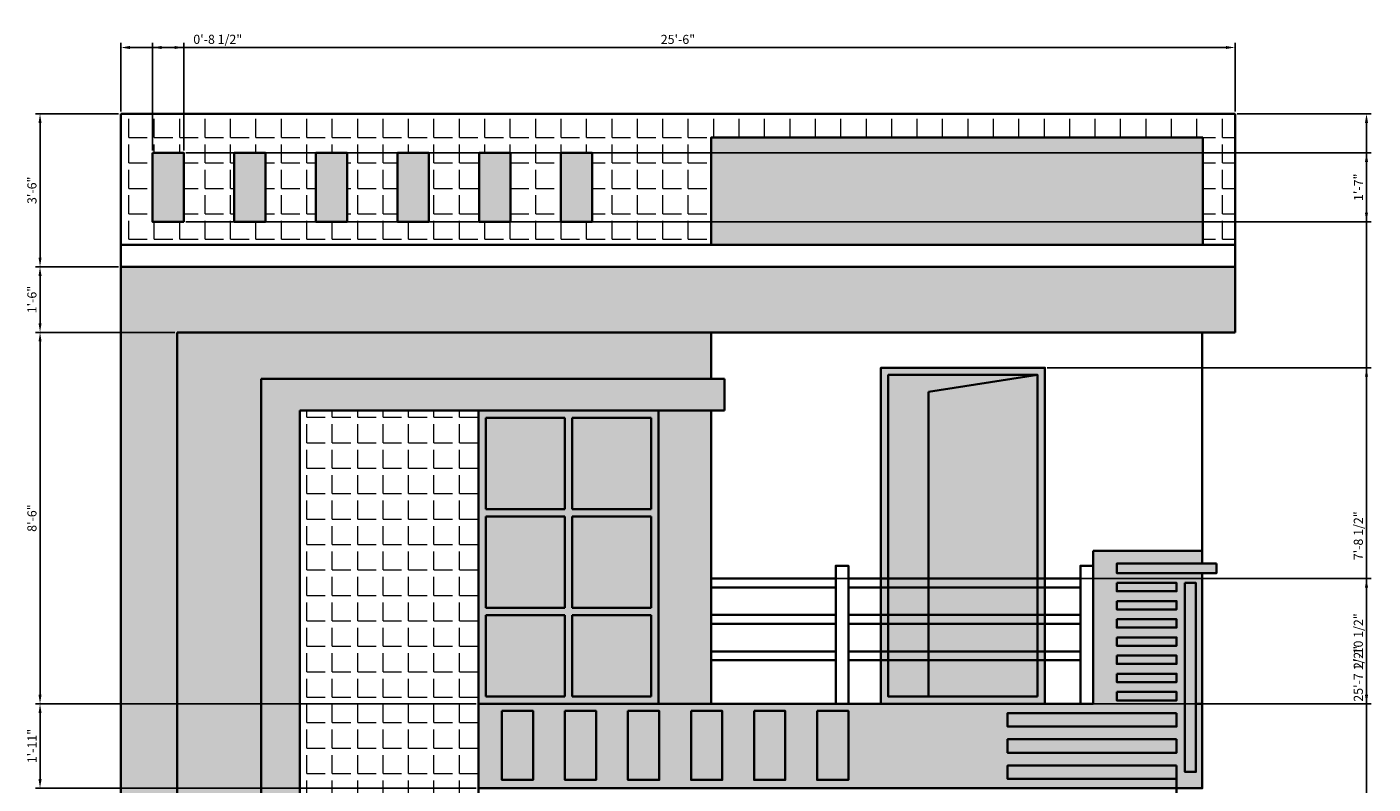
# Model space of a CAD drawing. Units: inches. Extents: x 2117 to 3047, y 1240 to 2266.
# Tile 3 of 4: x 2214 to 2584, y 2058 to 2266. Entities that reach past the tile are written whole.
import ezdxf

# ---------------------------------------------------------------- set-up
doc = ezdxf.new("R2010")
doc.units = ezdxf.units.IN
for name, color, linetype, lineweight in [('A-ANNO-DIMS', 2, 'Continuous', 18), ('A-ELEV', 7, 'Continuous', 35), ('A-ELEV-PATT', 8, 'Continuous', 13)]:
    doc.layers.add(name, color=color, linetype=linetype, lineweight=lineweight)
doc.styles.get("Standard").update_dxf_attribs({"font": 'arial.ttf'})
doc.dimstyles.new('ISO-25', dxfattribs={"dimtxt": 2.5, "dimasz": 2.5, "dimexe": 1.25, "dimexo": 0.625, "dimtad": 1, "dimdec": 1, "dimlunit": 3, "dimtxsty": 'Standard', "dimcen": 2.5, "dimadec": 0, "dimazin": 0, "dimtfac": 1, "dimtdec": 1, "dimtmove": 0, "dimatfit": 3, "dimfxl": 1, "dimarcsym": 0})
pattern_1 = [(0, (0, 0), (0, 6.985), [5.08, -1.905]), (90, (0, 0), (-6.985, 4e-16), [5.08, -1.905])]

# ---------------------------------------------------------------- blocks, each defined once
blk = doc.blocks.new('*D40')
at = {"layer": 'A-ANNO-DIMS', "color": 0, "lineweight": -2, "transparency": 16777216}
for p, q in [((2240.01, 2242.33), (2240.01, 2261.15)), ((2242.51, 2259.9), (2543.51, 2259.9)), ((2546.01, 2242.33), (2546.01, 2261.15))]:
    blk.add_line(p, q, dxfattribs=at)
at = {"layer": 'A-ANNO-DIMS', "color": 0, "transparency": 16777216}
for points in [[(2242.51, 2260.32), (2242.51, 2259.48), (2240.01, 2259.9)], [(2543.51, 2260.32), (2543.51, 2259.48), (2546.01, 2259.9)]]:
    blk.add_solid(points, dxfattribs=at)
at = {"layer": 'Defpoints', "color": 0, "transparency": 16777216}
for p in [(2546.01, 2259.9), (2240.01, 2241.7), (2546.01, 2241.7)]:
    blk.add_point(p, dxfattribs=at)
at = {"layer": 'A-ANNO-DIMS', "color": 0, "transparency": 16777216, "insert": (2393.01, 2261.8), "char_height": 2.5, "attachment_point": 5}
blk.add_mtext('25\'-6"', dxfattribs=at)
blk = doc.blocks.new('*D41')
at = {"layer": 'A-ANNO-DIMS', "color": 0, "lineweight": -2, "transparency": 16777216}
for p, q in [((2248.68, 2231.63), (2248.68, 2261.15)), ((2251.18, 2259.9), (2254.76, 2259.9)), ((2257.26, 2231.63), (2257.26, 2261.15)), ((2257.26, 2259.9), (2273.48, 2259.9))]:
    blk.add_line(p, q, dxfattribs=at)
at = {"layer": 'A-ANNO-DIMS', "color": 0, "transparency": 16777216}
for points in [[(2251.18, 2260.32), (2251.18, 2259.48), (2248.68, 2259.9)], [(2254.76, 2260.32), (2254.76, 2259.48), (2257.26, 2259.9)]]:
    blk.add_solid(points, dxfattribs=at)
at = {"layer": 'Defpoints', "color": 0, "transparency": 16777216}
for p in [(2257.26, 2259.9), (2248.68, 2231), (2257.26, 2231)]:
    blk.add_point(p, dxfattribs=at)
at = {"layer": 'A-ANNO-DIMS', "color": 0, "transparency": 16777216, "insert": (2266.62, 2261.82), "char_height": 2.5, "attachment_point": 5}
blk.add_mtext('0\'-8 1/2"', dxfattribs=at)
blk = doc.blocks.new('*D44')
at = {"layer": 'A-ANNO-DIMS', "color": 0, "lineweight": -2, "transparency": 16777216}
for p, q in [((2337.6, 2079.7), (2216.56, 2079.7)), ((2217.81, 2059.04), (2217.81, 2077.2)), ((2337.6, 2056.54), (2216.56, 2056.54))]:
    blk.add_line(p, q, dxfattribs=at)
at = {"layer": 'A-ANNO-DIMS', "color": 0, "transparency": 16777216}
for points in [[(2217.4, 2077.2), (2218.23, 2077.2), (2217.81, 2079.7)], [(2217.4, 2059.04), (2218.23, 2059.04), (2217.81, 2056.54)]]:
    blk.add_solid(points, dxfattribs=at)
at = {"layer": 'Defpoints', "color": 0, "transparency": 16777216}
for p in [(2217.81, 2079.7), (2338.23, 2079.7), (2338.23, 2056.54)]:
    blk.add_point(p, dxfattribs=at)
at = {"layer": 'A-ANNO-DIMS', "color": 0, "transparency": 16777216, "insert": (2215.93, 2068.12), "char_height": 2.5, "attachment_point": 5, "rotation": 90}
blk.add_mtext('1\'-11"', dxfattribs=at)
blk = doc.blocks.new('*D45')
at = {"layer": 'A-ANNO-DIMS', "color": 0, "lineweight": -2, "transparency": 16777216}
for p, q in [((2254.8, 2181.7), (2216.56, 2181.7)), ((2217.81, 2082.2), (2217.81, 2179.2)), ((2337.6, 2079.7), (2216.56, 2079.7))]:
    blk.add_line(p, q, dxfattribs=at)
at = {"layer": 'A-ANNO-DIMS', "color": 0, "transparency": 16777216}
for points in [[(2217.4, 2179.2), (2218.23, 2179.2), (2217.81, 2181.7)], [(2217.4, 2082.2), (2218.23, 2082.2), (2217.81, 2079.7)]]:
    blk.add_solid(points, dxfattribs=at)
at = {"layer": 'Defpoints', "color": 0, "transparency": 16777216}
for p in [(2217.81, 2181.7), (2255.43, 2181.7), (2338.23, 2079.7)]:
    blk.add_point(p, dxfattribs=at)
at = {"layer": 'A-ANNO-DIMS', "color": 0, "transparency": 16777216, "insert": (2215.91, 2130.7), "char_height": 2.5, "attachment_point": 5, "rotation": 90}
blk.add_mtext('8\'-6"', dxfattribs=at)
blk = doc.blocks.new('*D46')
at = {"layer": 'A-ANNO-DIMS', "color": 0, "lineweight": -2, "transparency": 16777216}
for p, q in [((2239.39, 2199.7), (2216.56, 2199.7)), ((2217.81, 2184.2), (2217.81, 2197.2)), ((2254.8, 2181.7), (2216.56, 2181.7))]:
    blk.add_line(p, q, dxfattribs=at)
at = {"layer": 'A-ANNO-DIMS', "color": 0, "transparency": 16777216}
for points in [[(2217.4, 2197.2), (2218.23, 2197.2), (2217.81, 2199.7)], [(2217.4, 2184.2), (2218.23, 2184.2), (2217.81, 2181.7)]]:
    blk.add_solid(points, dxfattribs=at)
at = {"layer": 'Defpoints', "color": 0, "transparency": 16777216}
for p in [(2217.81, 2199.7), (2240.01, 2199.7), (2255.43, 2181.7)]:
    blk.add_point(p, dxfattribs=at)
at = {"layer": 'A-ANNO-DIMS', "color": 0, "transparency": 16777216, "insert": (2215.91, 2190.7), "char_height": 2.5, "attachment_point": 5, "rotation": 90}
blk.add_mtext('1\'-6"', dxfattribs=at)
blk = doc.blocks.new('*D47')
at = {"layer": 'A-ANNO-DIMS', "color": 0, "lineweight": -2, "transparency": 16777216}
for p, q in [((2239.39, 2241.7), (2216.56, 2241.7)), ((2217.81, 2202.2), (2217.81, 2239.2)), ((2239.39, 2199.7), (2216.56, 2199.7))]:
    blk.add_line(p, q, dxfattribs=at)
at = {"layer": 'A-ANNO-DIMS', "color": 0, "transparency": 16777216}
for points in [[(2217.4, 2239.2), (2218.23, 2239.2), (2217.81, 2241.7)], [(2217.4, 2202.2), (2218.23, 2202.2), (2217.81, 2199.7)]]:
    blk.add_solid(points, dxfattribs=at)
at = {"layer": 'Defpoints', "color": 0, "transparency": 16777216}
for p in [(2217.81, 2241.7), (2240.01, 2241.7), (2240.01, 2199.7)]:
    blk.add_point(p, dxfattribs=at)
at = {"layer": 'A-ANNO-DIMS', "color": 0, "transparency": 16777216, "insert": (2215.91, 2220.7), "char_height": 2.5, "attachment_point": 5, "rotation": 90}
blk.add_mtext('3\'-6"', dxfattribs=at)
blk = doc.blocks.new('*D48')
at = {"layer": 'A-ANNO-DIMS', "color": 0, "lineweight": -2, "transparency": 16777216}
for p, q in [((2546.64, 2241.7), (2583.37, 2241.7)), ((2582.12, 1936.7), (2582.12, 2239.2)), ((2564.54, 1934.2), (2583.37, 1934.2))]:
    blk.add_line(p, q, dxfattribs=at)
at = {"layer": 'A-ANNO-DIMS', "color": 0, "transparency": 16777216}
for points in [[(2581.7, 2239.2), (2582.54, 2239.2), (2582.12, 2241.7)], [(2581.7, 1936.7), (2582.54, 1936.7), (2582.12, 1934.2)]]:
    blk.add_solid(points, dxfattribs=at)
at = {"layer": 'Defpoints', "color": 0, "transparency": 16777216}
for p in [(2546.01, 2241.7), (2582.12, 2241.7), (2563.92, 1934.2)]:
    blk.add_point(p, dxfattribs=at)
at = {"layer": 'A-ANNO-DIMS', "color": 0, "transparency": 16777216, "insert": (2580.2, 2087.95), "char_height": 2.5, "attachment_point": 5, "rotation": 90}
blk.add_mtext('25\'-7 1/2"', dxfattribs=at)
blk = doc.blocks.new('*D50')
at = {"layer": 'A-ANNO-DIMS', "color": 0, "lineweight": -2, "transparency": 16777216}
for p, q in [((2494.42, 2172), (2583.37, 2172)), ((2582.12, 2082.2), (2582.12, 2169.5)), ((2494.42, 2079.7), (2583.37, 2079.7))]:
    blk.add_line(p, q, dxfattribs=at)
at = {"layer": 'A-ANNO-DIMS', "color": 0, "transparency": 16777216}
for points in [[(2581.7, 2169.5), (2582.54, 2169.5), (2582.12, 2172)], [(2581.7, 2082.2), (2582.54, 2082.2), (2582.12, 2079.7)]]:
    blk.add_solid(points, dxfattribs=at)
at = {"layer": 'Defpoints', "color": 0, "transparency": 16777216}
for p in [(2493.8, 2172), (2582.12, 2172), (2493.8, 2079.7)]:
    blk.add_point(p, dxfattribs=at)
at = {"layer": 'A-ANNO-DIMS', "color": 0, "transparency": 16777216, "insert": (2580.2, 2125.85), "char_height": 2.5, "attachment_point": 5, "rotation": 90}
blk.add_mtext('7\'-8 1/2"', dxfattribs=at)
blk = doc.blocks.new('*D51')
at = {"layer": 'A-ANNO-DIMS', "color": 0, "lineweight": -2, "transparency": 16777216}
for p, q in [((2402.75, 2114.12), (2583.37, 2114.12)), ((2582.12, 2082.2), (2582.12, 2111.62)), ((2402.75, 2079.7), (2583.37, 2079.7))]:
    blk.add_line(p, q, dxfattribs=at)
at = {"layer": 'A-ANNO-DIMS', "color": 0, "transparency": 16777216}
for points in [[(2581.7, 2111.62), (2582.54, 2111.62), (2582.12, 2114.12)], [(2581.7, 2082.2), (2582.54, 2082.2), (2582.12, 2079.7)]]:
    blk.add_solid(points, dxfattribs=at)
at = {"layer": 'Defpoints', "color": 0, "transparency": 16777216}
for p in [(2402.12, 2114.12), (2582.12, 2114.12), (2402.12, 2079.7)]:
    blk.add_point(p, dxfattribs=at)
at = {"layer": 'A-ANNO-DIMS', "color": 0, "transparency": 16777216, "insert": (2580.2, 2096.91), "char_height": 2.5, "attachment_point": 5, "rotation": 90}
blk.add_mtext('2\'-10 1/2"', dxfattribs=at)
blk = doc.blocks.new('*D53')
at = {"layer": 'A-ANNO-DIMS', "color": 0, "lineweight": -2, "transparency": 16777216}
for p, q in [((2257.88, 2231), (2583.37, 2231)), ((2582.12, 2214.56), (2582.12, 2228.5)), ((2257.88, 2212.06), (2583.37, 2212.06))]:
    blk.add_line(p, q, dxfattribs=at)
at = {"layer": 'A-ANNO-DIMS', "color": 0, "transparency": 16777216}
for points in [[(2581.7, 2228.5), (2582.54, 2228.5), (2582.12, 2231)], [(2581.7, 2214.56), (2582.54, 2214.56), (2582.12, 2212.06)]]:
    blk.add_solid(points, dxfattribs=at)
at = {"layer": 'Defpoints', "color": 0, "transparency": 16777216}
for p in [(2257.26, 2231), (2582.12, 2231), (2257.26, 2212.06)]:
    blk.add_point(p, dxfattribs=at)
at = {"layer": 'A-ANNO-DIMS', "color": 0, "transparency": 16777216, "insert": (2580.24, 2221.53), "char_height": 2.5, "attachment_point": 5, "rotation": 90}
blk.add_mtext('1\'-7"', dxfattribs=at)

msp = doc.modelspace()

# ---------------------------------------------------------------- hatches: boundary and pattern name
at = {"layer": 'A-ELEV-PATT'}
h = msp.add_hatch(dxfattribs=at)
h.set_pattern_fill('ANGLE', color=256)
h.set_pattern_definition(pattern_1)
h.paths.add_polyline_path([(2402.12, 2235.15), (2537.18, 2235.15), (2537.18, 2205.7), (2546.01, 2205.7), (2546.01, 2241.7), (2240.01, 2241.7), (2240.01, 2205.7), (2402.12, 2205.7)])
h.paths.add_polyline_path([(2369.44, 2212.06), (2360.87, 2212.06), (2360.87, 2231), (2369.44, 2231)], flags=16)
h.paths.add_polyline_path([(2347, 2212.06), (2338.43, 2212.06), (2338.43, 2231), (2347, 2231)], flags=16)
h.paths.add_polyline_path([(2324.57, 2212.06), (2315.99, 2212.06), (2315.99, 2231), (2324.57, 2231)], flags=16)
h.paths.add_polyline_path([(2302.13, 2212.06), (2293.56, 2212.06), (2293.56, 2231), (2302.13, 2231)], flags=16)
h.paths.add_polyline_path([(2279.69, 2212.06), (2271.12, 2212.06), (2271.12, 2231), (2279.69, 2231)], flags=16)
h.paths.add_polyline_path([(2257.26, 2212.06), (2248.68, 2212.06), (2248.68, 2231), (2257.26, 2231)], flags=16)
h = msp.add_hatch(color=256, dxfattribs=at)
h.dxf.hatch_style = 1
h.paths.add_polyline_path([(2537.18, 2235.15), (2402.12, 2235.15), (2402.12, 2205.7), (2537.18, 2205.7)])
h = msp.add_hatch(color=256, dxfattribs=at)
h.dxf.hatch_style = 1
h.paths.add_polyline_path([(2257.26, 2231), (2248.68, 2231), (2248.68, 2212.06), (2257.26, 2212.06)])
h.paths.add_polyline_path([(2279.69, 2231), (2271.12, 2231), (2271.12, 2212.06), (2279.69, 2212.06)])
h.paths.add_polyline_path([(2293.56, 2212.06), (2302.13, 2212.06), (2302.13, 2231), (2293.56, 2231)])
h.paths.add_polyline_path([(2324.57, 2231), (2315.99, 2231), (2315.99, 2212.06), (2324.57, 2212.06)])
h.paths.add_polyline_path([(2347, 2231), (2338.43, 2231), (2338.43, 2212.06), (2347, 2212.06)])
h.paths.add_polyline_path([(2369.44, 2231), (2360.87, 2231), (2360.87, 2212.06), (2369.44, 2212.06)])
h = msp.add_hatch(color=256, dxfattribs=at)
h.dxf.hatch_style = 1
h.paths.add_polyline_path([(2248.68, 2212.06), (2257.26, 2212.06), (2257.26, 2231), (2248.68, 2231)])
h.paths.add_polyline_path([(2279.69, 2231), (2271.12, 2231), (2271.12, 2212.06), (2279.69, 2212.06)])
h.paths.add_polyline_path([(2293.56, 2212.06), (2302.13, 2212.06), (2302.13, 2231), (2293.56, 2231)])
h.paths.add_polyline_path([(2315.99, 2212.06), (2324.57, 2212.06), (2324.57, 2231), (2315.99, 2231)])
h.paths.add_polyline_path([(2338.43, 2212.06), (2347, 2212.06), (2347, 2231), (2338.43, 2231)])
h.paths.add_polyline_path([(2369.44, 2231), (2360.87, 2231), (2360.87, 2212.06), (2369.44, 2212.06)])
h = msp.add_hatch(dxfattribs=at)
h.set_pattern_fill('AR-CONC', color=256, scale=30)
h.set_pattern_definition([(50, (-387, -0.0008), (5465.5, -478), [571.5, -6286.5]), (355, (-387, -0.0008), (-1057.3, 5731.7), [457.2, -5029.2]), (100.45, (68.6, -40), (4408, 5253.5), [485.7, -5342.7]), (46.18, (-387, 1524), (8132.4, -1261), [857.2, -9429.8]), (96.64, (291, 1419), (7122, 7423), [728.6, -8014]), (351.18, (-387, 1524), (7122, 7423), [686, -7544]), (21, (375, 1143), (4548.4, -3068), [571.5, -6286.5]), (326, (375, 1143), (1854, 5525.6), [457.2, -5029.2]), (71.45, (754, 887.3), (6402.5, 2457.7), [485.7, -5342.7]), (37.5, (-386.8, -0.0008), (92.7, 2536.7), [0, -4968.24, 0, -5105.4, 0, -5048.25]), (7.5, (-386.8, -0.0008), (2004.6, 3005.4), [0, -2910.84, 0, -4853.94, 0, -1924.05]), (327.5, (-2086.1, -0.0008), (4067.7, -171.9), [0, -1905, 0, -5943.6, 0, -7886.7]), (317.5, (-2848, -0.0008), (4443.9, 762.8), [0, -2476.5, 0, -3947.2, 0, -5600.7])])
h.paths.add_polyline_path([(2249.02, 2199.7), (2537.02, 2199.7), (2537.02, 2175.7), (2546.02, 2175.7), (2546.02, 2205.7), (2240.02, 2205.7), (2240.02, 2175.7), (2249.02, 2175.7)])
h.paths.add_polyline_path([(2546.02, 2079.7), (2240.02, 2079.7), (2240.02, 2049.7), (2249.02, 2049.7), (2249.02, 2073.7), (2537.02, 2073.7), (2537.02, 2049.7), (2546.02, 2049.7)])
h = msp.add_hatch(color=256, dxfattribs=at)
h.dxf.hatch_style = 1
h.paths.add_polyline_path([(2537.01, 2199.7), (2240.01, 2199.7), (2240.01, 1953.7), (2255.43, 1953.7), (2255.43, 2181.7), (2537.01, 2181.7)])
h = msp.add_hatch(color=256, dxfattribs=at)
h.dxf.hatch_style = 1
h.paths.add_polyline_path([(2546.01, 2199.7), (2537.01, 2199.7), (2537.01, 2181.7), (2546.01, 2181.7)])
h = msp.add_hatch(color=256, dxfattribs=at)
h.dxf.hatch_style = 1
h.paths.add_polyline_path([(2278.52, 2168.93), (2402.12, 2168.93), (2402.12, 2181.7), (2255.43, 2181.7), (2255.43, 2079.7), (2278.52, 2079.7)])
h.paths.add_polyline_path([(2278.52, 2079.7), (2255.43, 2079.7), (2255.43, 2073.7), (2278.52, 2073.7)])
h.paths.add_polyline_path([(2278.52, 2073.7), (2255.43, 2073.7), (2255.43, 1953.7), (2278.52, 1953.7)])
h = msp.add_hatch(color=256, dxfattribs=at)
h.dxf.hatch_style = 1
h.paths.add_polyline_path([(2493.8, 2172), (2448.76, 2172), (2448.76, 2079.7), (2493.8, 2079.7)])
h.paths.add_polyline_path([(2491.8, 2170), (2491.8, 2081.7), (2450.76, 2081.7), (2450.76, 2170)], flags=16)
h.paths.add_polyline_path([(2491.8, 2170), (2461.79, 2165.39), (2461.79, 2081.7), (2491.8, 2081.7)], flags=0)
h = msp.add_hatch(color=256, dxfattribs=at)
h.dxf.hatch_style = 1
h.paths.add_polyline_path([(2289.19, 2160.2), (2405.83, 2160.2), (2405.83, 2168.93), (2402.12, 2168.93), (2278.52, 2168.93), (2278.52, 1953.7), (2289.19, 1953.7)])
h = msp.add_hatch(color=256, dxfattribs=at)
h.dxf.hatch_style = 1
h.paths.add_polyline_path([(2461.79, 2165.39), (2491.8, 2170), (2450.76, 2170), (2450.76, 2081.7), (2461.79, 2081.7)])
h = msp.add_hatch(color=256, dxfattribs=at)
h.dxf.hatch_style = 1
h.paths.add_polyline_path([(2491.8, 2170), (2461.79, 2165.39), (2461.79, 2081.7), (2491.8, 2081.7)])
h = msp.add_hatch(dxfattribs=at)
h.set_pattern_fill('ANGLE', color=256)
h.set_pattern_definition(pattern_1)
h.paths.add_polyline_path([(2338.23, 2160.2), (2289.19, 2160.2), (2289.19, 2079.7), (2338.23, 2079.7)])
h.paths.add_polyline_path([(2338.23, 2079.7), (2289.19, 2079.7), (2289.19, 2073.7), (2338.23, 2073.7)])
h = msp.add_hatch(dxfattribs=at)
h.set_pattern_fill('ANGLE', color=256)
h.set_pattern_definition(pattern_1)
h.paths.add_polyline_path([(2338.23, 2160.2), (2289.19, 2160.2), (2289.19, 1953.7), (2338.23, 1953.7)])
h = msp.add_hatch(color=256, dxfattribs=at)
h.dxf.hatch_style = 1
h.paths.add_polyline_path([(2363.93, 2158.2), (2361.93, 2158.2), (2361.93, 2133.13), (2361.93, 2131.13), (2361.93, 2106.05), (2361.93, 2104.05), (2361.93, 2081.7), (2361.93, 2079.7), (2363.93, 2079.7), (2363.93, 2131.13)])
h.paths.add_polyline_path([(2385.63, 2133.13), (2363.93, 2133.13), (2363.93, 2131.13), (2385.63, 2131.13)])
h.paths.add_polyline_path([(2361.93, 2133.13), (2340.23, 2133.13), (2340.23, 2131.13), (2361.93, 2131.13)])
h.paths.add_polyline_path([(2387.63, 2158.2), (2385.63, 2158.2), (2385.63, 2133.13), (2385.63, 2131.13), (2385.63, 2081.7), (2385.63, 2079.7), (2387.63, 2079.7)])
h.paths.add_polyline_path([(2385.63, 2106.05), (2363.93, 2106.05), (2363.93, 2104.05), (2385.63, 2104.05)])
h.paths.add_polyline_path([(2385.63, 2081.7), (2363.93, 2081.7), (2363.93, 2079.7), (2385.63, 2079.7)])
h.paths.add_polyline_path([(2361.93, 2081.7), (2340.23, 2081.7), (2340.23, 2079.7), (2361.93, 2079.7)])
h.paths.add_polyline_path([(2361.93, 2106.05), (2340.23, 2106.05), (2340.23, 2104.05), (2361.93, 2104.05)])
h.paths.add_polyline_path([(2387.63, 2160.2), (2338.23, 2160.2), (2338.23, 2158.2), (2340.23, 2158.2), (2361.93, 2158.2), (2363.93, 2158.2), (2385.63, 2158.2), (2387.63, 2158.2)])
h.paths.add_polyline_path([(2340.23, 2158.2), (2338.23, 2158.2), (2338.23, 2079.7), (2340.23, 2079.7), (2340.23, 2081.7), (2340.23, 2104.05), (2340.23, 2106.05), (2340.23, 2131.13), (2340.23, 2133.13)])
h = msp.add_hatch(color=256, dxfattribs=at)
h.dxf.hatch_style = 1
h.paths.add_polyline_path([(2402.12, 2160.2), (2387.63, 2160.2), (2387.63, 2079.7), (2393.1, 2079.7), (2402.12, 2079.7)])
h = msp.add_hatch(color=256, dxfattribs=at)
h.dxf.hatch_style = 1
h.paths.add_polyline_path([(2361.93, 2158.2), (2340.23, 2158.2), (2340.23, 2133.13), (2361.93, 2133.13)])
h.paths.add_polyline_path([(2385.63, 2158.2), (2363.93, 2158.2), (2363.93, 2133.13), (2385.63, 2133.13)])
h.paths.add_polyline_path([(2361.93, 2131.13), (2340.23, 2131.13), (2340.23, 2106.05), (2361.93, 2106.05)])
h.paths.add_polyline_path([(2385.63, 2131.13), (2363.93, 2131.13), (2363.93, 2106.05), (2385.63, 2106.05)])
h.paths.add_polyline_path([(2361.93, 2104.05), (2340.23, 2104.05), (2340.23, 2081.7), (2361.93, 2081.7)])
h.paths.add_polyline_path([(2385.63, 2104.05), (2363.93, 2104.05), (2363.93, 2081.7), (2385.63, 2081.7)])
h = msp.add_hatch(color=256, dxfattribs=at)
h.dxf.hatch_style = 1
h.paths.add_polyline_path([(2537.01, 2115.61), (2513.52, 2115.61), (2513.52, 2118.22), (2537.01, 2118.22), (2537.01, 2121.7), (2507.01, 2121.7), (2507.01, 2079.7), (2532.24, 2079.7), (2532.24, 2112.91), (2535.26, 2112.91), (2535.26, 2079.7), (2537.01, 2079.7)])
h.paths.add_polyline_path([(2513.52, 2112.91), (2529.98, 2112.91), (2529.98, 2110.61), (2513.52, 2110.61)], flags=16)
h.paths.add_polyline_path([(2513.52, 2107.91), (2529.98, 2107.91), (2529.98, 2105.62), (2513.52, 2105.62)], flags=16)
h.paths.add_polyline_path([(2513.52, 2102.92), (2529.98, 2102.92), (2529.98, 2100.63), (2513.52, 2100.63)], flags=16)
h.paths.add_polyline_path([(2513.52, 2097.93), (2529.98, 2097.93), (2529.98, 2095.64), (2513.52, 2095.64)], flags=16)
h.paths.add_polyline_path([(2513.52, 2092.94), (2529.98, 2092.94), (2529.98, 2090.65), (2513.52, 2090.65)], flags=16)
h.paths.add_polyline_path([(2513.52, 2087.95), (2529.98, 2087.95), (2529.98, 2085.66), (2513.52, 2085.66)], flags=16)
h.paths.add_polyline_path([(2513.52, 2082.96), (2529.98, 2082.96), (2529.98, 2080.67), (2513.52, 2080.67)], flags=16)
h = msp.add_hatch(color=256, dxfattribs=at)
h.dxf.hatch_style = 1
h.paths.add_polyline_path([(2537.01, 2118.22), (2513.52, 2118.22), (2513.52, 2115.61), (2537.01, 2115.61)])
h.paths.add_polyline_path([(2540.95, 2118.22), (2537.01, 2118.22), (2537.01, 2115.61), (2540.95, 2115.61)])
h.paths.add_polyline_path([(2529.98, 2112.91), (2513.52, 2112.91), (2513.52, 2110.61), (2529.98, 2110.61)])
h.paths.add_polyline_path([(2529.98, 2107.91), (2513.52, 2107.91), (2513.52, 2105.62), (2529.98, 2105.62)])
h.paths.add_polyline_path([(2529.98, 2102.92), (2513.52, 2102.92), (2513.52, 2100.63), (2529.98, 2100.63)])
h.paths.add_polyline_path([(2529.98, 2097.93), (2513.52, 2097.93), (2513.52, 2095.64), (2529.98, 2095.64)])
h.paths.add_polyline_path([(2529.98, 2092.94), (2513.52, 2092.94), (2513.52, 2090.65), (2529.98, 2090.65)])
h.paths.add_polyline_path([(2529.98, 2087.95), (2513.52, 2087.95), (2513.52, 2085.66), (2529.98, 2085.66)])
h.paths.add_polyline_path([(2529.98, 2082.96), (2513.52, 2082.96), (2513.52, 2080.67), (2529.98, 2080.67)])
h.paths.add_polyline_path([(2535.26, 2112.91), (2532.24, 2112.91), (2532.24, 2079.7), (2535.26, 2079.7)])
h.paths.add_polyline_path([(2387.86, 2077.77), (2379.29, 2077.77), (2379.29, 2058.82), (2387.86, 2058.82)])
h.paths.add_polyline_path([(2370.54, 2077.77), (2361.97, 2077.77), (2361.97, 2058.82), (2370.54, 2058.82)])
h.paths.add_polyline_path([(2353.23, 2077.77), (2344.66, 2077.77), (2344.66, 2058.82), (2353.23, 2058.82)])
h.paths.add_polyline_path([(2405.18, 2077.77), (2396.61, 2077.77), (2396.61, 2058.82), (2405.18, 2058.82)])
h.paths.add_polyline_path([(2422.49, 2077.77), (2413.92, 2077.77), (2413.92, 2058.82), (2422.49, 2058.82)])
h.paths.add_polyline_path([(2439.81, 2077.77), (2431.24, 2077.77), (2431.24, 2058.82), (2439.81, 2058.82)])
h.paths.add_polyline_path([(2529.98, 2077.15), (2483.54, 2077.15), (2483.54, 2073.48), (2529.98, 2073.48)])
h.paths.add_polyline_path([(2529.98, 2069.97), (2483.54, 2069.97), (2483.54, 2066.3), (2529.98, 2066.3)])
h.paths.add_polyline_path([(2529.98, 2062.78), (2483.54, 2062.78), (2483.54, 2059.12), (2529.98, 2059.12)])
h.paths.add_polyline_path([(2535.26, 2079.7), (2532.24, 2079.7), (2532.24, 2061), (2535.26, 2061)])
h = msp.add_hatch(color=256, dxfattribs=at)
h.dxf.hatch_style = 1
h.paths.add_polyline_path([(2529.98, 2077.15), (2483.54, 2077.15), (2483.54, 2073.48), (2529.98, 2073.48)])
h.paths.add_polyline_path([(2529.98, 2069.97), (2483.54, 2069.97), (2483.54, 2066.3), (2529.98, 2066.3)])
h.paths.add_polyline_path([(2529.98, 2062.78), (2483.54, 2062.78), (2483.54, 2059.12), (2529.98, 2059.12)])
h.paths.add_polyline_path([(2535.26, 2112.91), (2532.24, 2112.91), (2532.24, 2079.7), (2535.26, 2079.7)])
h = msp.add_hatch(color=256, dxfattribs=at)
h.dxf.hatch_style = 1
h.paths.add_polyline_path([(2338.23, 2079.7), (2338.23, 2056.54), (2537.01, 2056.54), (2537.01, 2079.7), (2535.26, 2079.7), (2535.26, 2061), (2532.24, 2061), (2532.24, 2079.7)])
h.paths.add_polyline_path([(2529.98, 2077.15), (2529.98, 2073.48), (2483.54, 2073.48), (2483.54, 2077.15)], flags=16)
h.paths.add_polyline_path([(2529.98, 2069.97), (2529.98, 2066.3), (2483.54, 2066.3), (2483.54, 2069.97)], flags=16)
h.paths.add_polyline_path([(2529.98, 2062.78), (2529.98, 2059.12), (2483.54, 2059.12), (2483.54, 2062.78)], flags=16)
h.paths.add_polyline_path([(2439.81, 2077.77), (2439.81, 2058.82), (2431.24, 2058.82), (2431.24, 2077.77)], flags=16)
h.paths.add_polyline_path([(2422.49, 2077.77), (2422.49, 2058.82), (2413.92, 2058.82), (2413.92, 2077.77)], flags=16)
h.paths.add_polyline_path([(2405.18, 2077.77), (2405.18, 2058.82), (2396.61, 2058.82), (2396.61, 2077.77)], flags=16)
h.paths.add_polyline_path([(2387.86, 2077.77), (2387.86, 2058.82), (2379.29, 2058.82), (2379.29, 2077.77)], flags=16)
h.paths.add_polyline_path([(2370.54, 2077.77), (2370.54, 2058.82), (2361.97, 2058.82), (2361.97, 2077.77)], flags=16)
h.paths.add_polyline_path([(2353.23, 2077.77), (2353.23, 2058.82), (2344.66, 2058.82), (2344.66, 2077.77)], flags=16)

# ---------------------------------------------------------------- linework, layer by layer
at = {"layer": 'A-ELEV'}
for p, q in [((2240.01, 2241.7), (2546.01, 2241.7)), ((2240.01, 1949.2), (2240.01, 2241.7)), ((2546.01, 2181.7), (2546.01, 2241.7)), ((2240.01, 2205.7), (2546.01, 2205.7)), ((2240.01, 2199.7), (2546.01, 2199.7)), ((2546.01, 2199.7), (2546.01, 2187.7)), ((2546.01, 2199.7), (2546.01, 2181.7)), ((2546.01, 2181.7), (2255.43, 2181.7)), ((2255.43, 2181.7), (2255.43, 1953.7)), ((2402.12, 2181.7), (2402.12, 2168.93)), ((2537.01, 2118.22), (2537.01, 2181.7)), ((2402.12, 2168.93), (2278.52, 2168.93)), ((2278.52, 2168.93), (2278.52, 1953.7)), ((2402.12, 2168.93), (2405.83, 2168.93)), ((2405.83, 2168.93), (2405.83, 2160.2)), ((2491.8, 2170), (2461.79, 2165.39)), ((2461.79, 2165.39), (2461.79, 2081.7)), ((2405.83, 2160.2), (2289.19, 2160.2)), ((2289.19, 2160.2), (2289.19, 1953.7)), ((2338.23, 2160.2), (2338.23, 1953.7)), ((2338.23, 2160.2), (2405.83, 2160.2)), ((2338.23, 2160.2), (2405.83, 2160.2)), ((2387.63, 2160.2), (2338.23, 2160.2)), ((2338.23, 2160.2), (2338.23, 2079.7)), ((2387.63, 2079.7), (2387.63, 2160.2)), ((2402.12, 2160.2), (2402.12, 2079.7)), ((2340.23, 2158.2), (2340.23, 2133.13)), ((2361.93, 2158.2), (2340.23, 2158.2)), ((2361.93, 2158.2), (2361.93, 2133.13)), ((2363.93, 2158.2), (2363.93, 2133.13)), ((2363.93, 2158.2), (2363.93, 2133.13)), ((2385.63, 2158.2), (2363.93, 2158.2)), ((2363.93, 2158.2), (2363.93, 2133.13)), ((2385.63, 2133.13), (2385.63, 2158.2)), ((2361.93, 2133.13), (2340.23, 2133.13)), ((2361.93, 2131.13), (2340.23, 2131.13)), ((2340.23, 2131.13), (2340.23, 2106.05)), ((2361.93, 2131.13), (2361.93, 2106.05)), ((2385.63, 2133.13), (2363.93, 2133.13)), ((2385.63, 2131.13), (2363.93, 2131.13)), ((2363.93, 2131.13), (2363.93, 2106.05)), ((2363.93, 2131.13), (2363.93, 2106.05)), ((2363.93, 2131.13), (2363.93, 2106.05)), ((2385.63, 2106.05), (2385.63, 2131.13)), ((2537.01, 2118.22), (2537.01, 2127.7)), ((2537.01, 2118.22), (2537.01, 2127.7)), ((2537.01, 2121.7), (2507.01, 2121.7)), ((2507.01, 2121.7), (2507.01, 2079.7)), ((2537.01, 2118.22), (2537.01, 2121.7)), ((2537.01, 2079.7), (2537.01, 2115.61)), ((2537.01, 2079.7), (2537.01, 2115.61)), ((2537.01, 2079.7), (2537.01, 2115.61)), ((2537.01, 2079.7), (2537.01, 2115.61)), ((2361.93, 2106.05), (2340.23, 2106.05)), ((2340.23, 2104.05), (2340.23, 2081.7)), ((2361.93, 2104.05), (2340.23, 2104.05)), ((2361.93, 2104.05), (2361.93, 2081.7)), ((2385.63, 2106.05), (2363.93, 2106.05)), ((2385.63, 2104.05), (2363.93, 2104.05)), ((2363.93, 2104.05), (2363.93, 2081.7)), ((2363.93, 2104.05), (2363.93, 2081.7)), ((2363.93, 2104.05), (2363.93, 2081.7)), ((2385.63, 2081.7), (2385.63, 2104.05)), ((2340.23, 2081.7), (2361.93, 2081.7)), ((2363.93, 2081.7), (2385.63, 2081.7)), ((2338.23, 2079.7), (2367.44, 2079.7)), ((2338.23, 2079.7), (2387.63, 2079.7)), ((2363.93, 2079.7), (2361.93, 2079.7)), ((2535.26, 2079.7), (2537.01, 2079.7)), ((2529.98, 2059.12), (2529.98, 1953.7))]:
    msp.add_line(p, q, dxfattribs=at)
for points in [[(2537.18, 2235.15), (2402.12, 2235.15), (2402.12, 2205.7), (2537.18, 2205.7)], [(2248.68, 2231), (2257.26, 2231), (2257.26, 2212.06), (2248.68, 2212.06)], [(2271.12, 2231), (2279.69, 2231), (2279.69, 2212.06), (2271.12, 2212.06)], [(2293.56, 2231), (2302.13, 2231), (2302.13, 2212.06), (2293.56, 2212.06)], [(2315.99, 2231), (2324.57, 2231), (2324.57, 2212.06), (2315.99, 2212.06)], [(2338.43, 2231), (2347, 2231), (2347, 2212.06), (2338.43, 2212.06)], [(2360.87, 2231), (2369.44, 2231), (2369.44, 2212.06), (2360.87, 2212.06)], [(2493.8, 2079.7), (2448.76, 2079.7), (2448.76, 2172), (2493.8, 2172)], [(2491.8, 2081.7), (2450.76, 2081.7), (2450.76, 2170), (2491.8, 2170)], [(2540.95, 2118.22), (2513.52, 2118.22), (2513.52, 2115.61), (2540.95, 2115.61)], [(2513.52, 2112.91), (2529.98, 2112.91), (2529.98, 2110.61), (2513.52, 2110.61)], [(2532.24, 2112.91), (2535.26, 2112.91), (2535.26, 2061), (2532.24, 2061)], [(2513.52, 2107.91), (2529.98, 2107.91), (2529.98, 2105.62), (2513.52, 2105.62)], [(2513.52, 2102.92), (2529.98, 2102.92), (2529.98, 2100.63), (2513.52, 2100.63)], [(2513.52, 2097.93), (2529.98, 2097.93), (2529.98, 2095.64), (2513.52, 2095.64)], [(2513.52, 2092.94), (2529.98, 2092.94), (2529.98, 2090.65), (2513.52, 2090.65)], [(2513.52, 2087.95), (2529.98, 2087.95), (2529.98, 2085.66), (2513.52, 2085.66)], [(2513.52, 2082.96), (2529.98, 2082.96), (2529.98, 2080.67), (2513.52, 2080.67)], [(2338.23, 2079.7), (2393.1, 2079.7), (2393.1, 2079.7), (2338.23, 2079.7)], [(2344.66, 2077.77), (2353.23, 2077.77), (2353.23, 2058.82), (2344.66, 2058.82)], [(2344.66, 2077.77), (2353.23, 2077.77), (2353.23, 2058.82), (2344.66, 2058.82)], [(2344.66, 2077.77), (2353.23, 2077.77), (2353.23, 2058.82), (2344.66, 2058.82)], [(2344.66, 2077.77), (2353.23, 2077.77), (2353.23, 2058.82), (2344.66, 2058.82)], [(2344.66, 2077.77), (2353.23, 2077.77), (2353.23, 2058.82), (2344.66, 2058.82)], [(2344.66, 2077.77), (2353.23, 2077.77), (2353.23, 2058.82), (2344.66, 2058.82)], [(2361.97, 2077.77), (2370.54, 2077.77), (2370.54, 2058.82), (2361.97, 2058.82)], [(2379.29, 2077.77), (2387.86, 2077.77), (2387.86, 2058.82), (2379.29, 2058.82)], [(2396.61, 2077.77), (2405.18, 2077.77), (2405.18, 2058.82), (2396.61, 2058.82)], [(2413.92, 2077.77), (2422.49, 2077.77), (2422.49, 2058.82), (2413.92, 2058.82)], [(2431.24, 2077.77), (2439.81, 2077.77), (2439.81, 2058.82), (2431.24, 2058.82)], [(2529.98, 2077.15), (2483.54, 2077.15), (2483.54, 2073.48), (2529.98, 2073.48)], [(2529.98, 2069.97), (2483.54, 2069.97), (2483.54, 2066.3), (2529.98, 2066.3)], [(2529.98, 2062.78), (2483.54, 2062.78), (2483.54, 2059.12), (2529.98, 2059.12)]]:
    msp.add_lwpolyline(points, close=True, dxfattribs=at)
for points in [[(2436.37, 2079.7), (2436.37, 2117.64), (2439.81, 2117.64), (2439.81, 2079.7)], [(2503.57, 2079.7), (2503.57, 2117.64), (2507.01, 2117.64), (2507.01, 2079.7)], [(2503.57, 2079.7), (2503.57, 2117.64), (2507.01, 2117.64), (2507.01, 2079.7)], [(2503.57, 2079.7), (2503.57, 2117.64), (2507.01, 2117.64), (2507.01, 2079.7)], [(2503.57, 2079.7), (2503.57, 2117.64), (2507.01, 2117.64), (2507.01, 2079.7)], [(2503.57, 2079.7), (2503.57, 2117.64), (2507.01, 2117.64), (2507.01, 2079.7)], [(2503.57, 2079.7), (2503.57, 2117.64), (2507.01, 2117.64), (2507.01, 2079.7)], [(2503.57, 2079.7), (2503.57, 2117.64), (2507.01, 2117.64), (2507.01, 2079.7)], [(2507.01, 2117.64), (2507.01, 2079.7)], [(2507.01, 2117.64), (2507.01, 2079.7)], [(2436.37, 2114.12), (2402.12, 2114.12), (2402.12, 2111.69), (2436.37, 2111.69)], [(2503.57, 2114.12), (2439.81, 2114.12)], [(2439.81, 2111.69), (2503.57, 2111.69)], [(2507.01, 2111.69), (2507.01, 2114.12)], [(2436.37, 2104.11), (2402.12, 2104.11), (2402.12, 2101.67), (2436.37, 2101.67)], [(2503.57, 2104.11), (2439.81, 2104.11)], [(2507.01, 2101.67), (2507.01, 2104.11)], [(2439.81, 2101.67), (2503.57, 2101.67)], [(2436.37, 2094.1), (2402.12, 2094.1), (2402.12, 2091.66), (2436.37, 2091.66)], [(2503.57, 2094.1), (2439.81, 2094.1)], [(2507.01, 2091.66), (2507.01, 2094.1)], [(2439.81, 2091.66), (2503.57, 2091.66)], [(2537.01, 2079.7), (2537.01, 2056.54), (2338.23, 2056.54), (2338.23, 2079.7), (2507.01, 2079.7)], [(2439.81, 2077.77), (2436.37, 2077.77)]]:
    msp.add_lwpolyline(points, dxfattribs=at)

# ---------------------------------------------------------------- dimensions: what is measured, and where the dimension line sits
at = {"layer": 'A-ANNO-DIMS'}
for base, p1, p2, picture, middle in [((2546.01, 2259.9), (2240.01, 2241.7), (2546.01, 2241.7), '*D40', (2393.01, 2261.8)), ((2257.26, 2259.9), (2248.68, 2231), (2257.26, 2231), '*D41', (2266.62, 2261.82))]:
    dim = msp.add_linear_dim(base=base, p1=p1, p2=p2, dimstyle='ISO-25', override={"dimdec": 1, "dimlfac": 1, "dimrnd": 0, "dimzin": 1, "dimdsep": 46, "dimlunit": 4, "dimfrac": 2}, dxfattribs=at)
    dim.commit()
    dim.dimension.update_dxf_attribs({"geometry": picture, "text_midpoint": middle})
for base, p1, p2, picture, middle in [((2217.81, 2241.7), (2240.01, 2199.7), (2240.01, 2241.7), '*D47', (2215.91, 2220.7)), ((2582.12, 2241.7), (2563.92, 1934.2), (2546.01, 2241.7), '*D48', (2580.2, 2087.95)), ((2582.12, 2231), (2257.26, 2212.06), (2257.26, 2231), '*D53', (2580.24, 2221.53)), ((2217.81, 2199.7), (2255.43, 2181.7), (2240.01, 2199.7), '*D46', (2215.91, 2190.7)), ((2217.81, 2181.7), (2338.23, 2079.7), (2255.43, 2181.7), '*D45', (2215.91, 2130.7)), ((2582.12, 2172), (2493.8, 2079.7), (2493.8, 2172), '*D50', (2580.2, 2125.85)), ((2582.12, 2114.12), (2402.12, 2079.7), (2402.12, 2114.12), '*D51', (2580.2, 2096.91)), ((2217.81, 2079.7), (2338.23, 2056.54), (2338.23, 2079.7), '*D44', (2215.93, 2068.12))]:
    dim = msp.add_linear_dim(base=base, p1=p1, p2=p2, angle=90, dimstyle='ISO-25', override={"dimdec": 1, "dimlfac": 1, "dimrnd": 0, "dimzin": 1, "dimdsep": 46, "dimlunit": 4, "dimfrac": 2}, dxfattribs=at)
    dim.commit()
    dim.dimension.update_dxf_attribs({"geometry": picture, "text_midpoint": middle})

doc.saveas('drawing.dxf')
